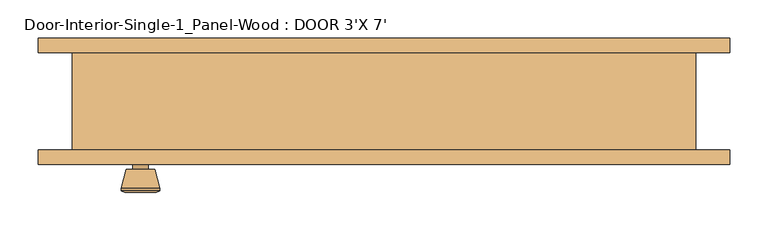
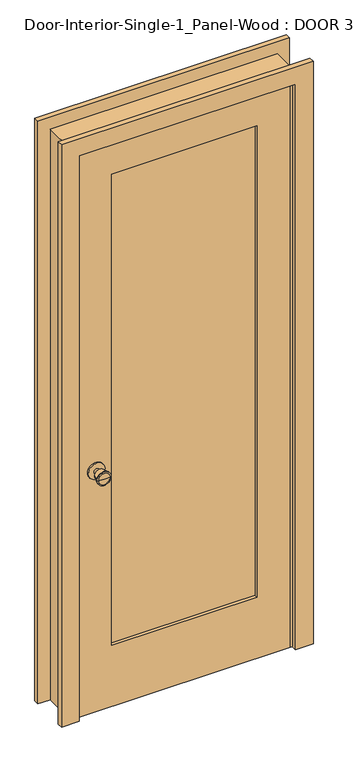
"""IFC4 building model written with IfcOpenShell, lengths in millimetres: door geometry, Door-Interior-Single-1_Panel-Wood : DOOR 3'X 7'."""

from ifc_helpers import new_model, si_unit, point, frame, frame_2d, origin, place, context, project, spatial, polyline, circle_curve, trimmed, segment, composite_curve, outline, extrude, faceted_brep, source, transform, mapped, element, save
from ifc_brep_helpers import plane_surface, cylinder_surface, revolved_surface, advanced_brep


def door_interior_single_1_panel_wood_door_3_x_7_fe7a9c6b(model_context):
    return source(origin(), model_context, "Body", "SolidModel", [
        advanced_brep(
        [(-317.5, -19.4, 914.4), (-327.5, -19.4, 914.4), (-307.5, -19.4, 914.4), (-297.0241324, 29.6, 914.4), (-337.9758676, 29.6, 914.4), (-317.5, 29.6, 914.4), (-292.5, 27.7721319, 914.4), (-342.5, 27.7721319, 914.4), (-292.5, 24.3084537, 914.4), (-342.5, 24.3084537, 914.4), (-298.863764, -0.4, 914.4), (-336.136236, -0.4, 914.4), (-307.5, -0.4, 914.4), (-327.5, -0.4, 914.4)],
        [
            (0, 1),
            (1, 2, circle_curve(frame((-317.5, -19.4, 914.4), z_axis=(0.0, -1.0, 0.0), x_axis=(-1.0, 0.0, 0.0)), 10.0)),
            (2, 0),
            (2, 1, circle_curve(frame((-317.5, -19.4, 914.4), z_axis=(0.0, -1.0, 0.0), x_axis=(-1.0, 0.0, 0.0)), 10.0)),
            (3, 4, circle_curve(frame((-317.5, 29.6, 914.4), z_axis=(0.0, 1.0, 0.0), x_axis=(-1.0, 0.0, 0.0)), 20.4758676)),
            (4, 5),
            (5, 3),
            (4, 3, circle_curve(frame((-317.5, 29.6, 914.4), z_axis=(0.0, 1.0, 0.0), x_axis=(-1.0, 0.0, 0.0)), 20.4758676)),
            (6, 7, circle_curve(frame((-317.5, 27.7721319, 914.4), z_axis=(0.0, 1.0, 0.0), x_axis=(-1.0, 0.0, 0.0)), 25.0)),
            (7, 4),
            (3, 6),
            (7, 6, circle_curve(frame((-317.5, 27.7721319, 914.4), z_axis=(0.0, 1.0, 0.0), x_axis=(-1.0, 0.0, 0.0)), 25.0)),
            (8, 9, circle_curve(frame((-317.5, 24.3084537, 914.4), z_axis=(0.0, 1.0, 0.0), x_axis=(-1.0, 0.0, 0.0)), 25.0)),
            (9, 7),
            (6, 8),
            (9, 8, circle_curve(frame((-317.5, 24.3084537, 914.4), z_axis=(0.0, 1.0, 0.0), x_axis=(-1.0, 0.0, 0.0)), 25.0)),
            (10, 11, circle_curve(frame((-317.5, -0.4, 914.4), z_axis=(0.0, 1.0, 0.0), x_axis=(-1.0, 0.0, 0.0)), 18.636236)),
            (11, 9),
            (8, 10),
            (11, 10, circle_curve(frame((-317.5, -0.4, 914.4), z_axis=(0.0, 1.0, 0.0), x_axis=(-1.0, 0.0, 0.0)), 18.636236)),
            (12, 13, circle_curve(frame((-317.5, -0.4, 914.4), z_axis=(0.0, 1.0, 0.0), x_axis=(-1.0, 0.0, 0.0)), 10.0)),
            (13, 11),
            (10, 12),
            (13, 12, circle_curve(frame((-317.5, -0.4, 914.4), z_axis=(0.0, 1.0, 0.0), x_axis=(-1.0, 0.0, 0.0)), 10.0)),
            (1, 13),
            (12, 2),
        ],
        [
            plane_surface(frame((-317.5, -19.4, 914.4), z_axis=(0.0, -1.0, 0.0), x_axis=(-1.0, 0.0, 0.0))),
            plane_surface(frame((-317.5, 29.6, 914.4), z_axis=(0.0, 1.0, 0.0), x_axis=(-1.0, 0.0, 0.0))),
            revolved_surface(polyline([(-337.9758676, 29.6, 914.4), (-342.5, 27.7721319, 914.4)]), (-317.5, -19.4, 914.4), (0.0, -1.0, 0.0)),
            cylinder_surface(frame((-317.5, -19.4, 914.4), z_axis=(0.0, -1.0, 0.0), x_axis=(-1.0, 0.0, 0.0)), 25.0),
            revolved_surface(polyline([(-342.5, 24.3084537, 914.4), (-336.136236, -0.4, 914.4)]), (-317.5, -19.4, 914.4), (0.0, -1.0, 0.0)),
            plane_surface(frame((-317.5, -0.4, 914.4), z_axis=(0.0, -1.0, 0.0), x_axis=(-1.0, 0.0, 0.0))),
            cylinder_surface(frame((-317.5, -19.4, 914.4), z_axis=(0.0, -1.0, 0.0), x_axis=(-1.0, 0.0, 0.0)), 10.0),
        ],
        [
            (0, [[1, 2, 3]]),
            (0, [[-3, 4, -1]]),
            (1, [[5, 6, 7]]),
            (1, [[8, -7, -6]]),
            (2, [[9, 10, -5, 11]]),
            (2, [[12, -11, -8, -10]]),
            (3, [[13, 14, -9, 15]]),
            (3, [[16, -15, -12, -14]]),
            (4, [[17, 18, -13, 19]]),
            (4, [[20, -19, -16, -18]]),
            (5, [[21, 22, -17, 23]]),
            (5, [[24, -23, -20, -22]]),
            (6, [[-2, 25, -21, 26]]),
            (6, [[-4, -26, -24, -25]]),
        ],
    ),
        extrude(outline(composite_curve([segment(trimmed(circle_curve(frame_2d((914.4, -317.5)), 30.0), [point((914.4, -347.5))], [point((914.4, -287.5))], False, "CARTESIAN"), True, "CONTINUOUS"), segment(trimmed(circle_curve(frame_2d((914.4, -317.5)), 30.0), [point((914.4, -287.5))], [point((914.4, -347.5))], False, "CARTESIAN"), True, "CONTINUOUS")], self_intersect=False)), frame((0.0, -25.4, 0.0), z_axis=(0.0, 1.0, 0.0), x_axis=(0.0, 0.0, 1.0)), (0.0, 0.0, 1.0), 6.0),
        advanced_brep(
        [(-317.5, -66.325, 914.4), (-307.5, -66.325, 914.4), (-327.5, -66.325, 914.4), (-297.0241324, -115.325, 914.4), (-317.5, -115.325, 914.4), (-337.9758676, -115.325, 914.4), (-292.5, -113.4971319, 914.4), (-342.5, -113.4971319, 914.4), (-292.5, -110.0334537, 914.4), (-342.5, -110.0334537, 914.4), (-298.863764, -85.325, 914.4), (-336.136236, -85.325, 914.4), (-307.5, -85.325, 914.4), (-327.5, -85.325, 914.4)],
        [
            (0, 1),
            (1, 2, circle_curve(frame((-317.5, -66.325, 914.4), z_axis=(0.0, 1.0, 0.0), x_axis=(-1.0, 0.0, 0.0)), 10.0)),
            (2, 0),
            (2, 1, circle_curve(frame((-317.5, -66.325, 914.4), z_axis=(0.0, 1.0, 0.0), x_axis=(-1.0, 0.0, 0.0)), 10.0)),
            (3, 4),
            (4, 5),
            (5, 3, circle_curve(frame((-317.5, -115.325, 914.4), z_axis=(0.0, -1.0, 0.0), x_axis=(-1.0, 0.0, 0.0)), 20.4758676)),
            (3, 5, circle_curve(frame((-317.5, -115.325, 914.4), z_axis=(0.0, -1.0, 0.0), x_axis=(-1.0, 0.0, 0.0)), 20.4758676)),
            (6, 3),
            (5, 7),
            (7, 6, circle_curve(frame((-317.5, -113.4971319, 914.4), z_axis=(0.0, -1.0, 0.0), x_axis=(-1.0, 0.0, 0.0)), 25.0)),
            (6, 7, circle_curve(frame((-317.5, -113.4971319, 914.4), z_axis=(0.0, -1.0, 0.0), x_axis=(-1.0, 0.0, 0.0)), 25.0)),
            (8, 6),
            (7, 9),
            (9, 8, circle_curve(frame((-317.5, -110.0334537, 914.4), z_axis=(0.0, -1.0, 0.0), x_axis=(-1.0, 0.0, 0.0)), 25.0)),
            (8, 9, circle_curve(frame((-317.5, -110.0334537, 914.4), z_axis=(0.0, -1.0, 0.0), x_axis=(-1.0, 0.0, 0.0)), 25.0)),
            (10, 8),
            (9, 11),
            (11, 10, circle_curve(frame((-317.5, -85.325, 914.4), z_axis=(0.0, -1.0, 0.0), x_axis=(-1.0, 0.0, 0.0)), 18.636236)),
            (10, 11, circle_curve(frame((-317.5, -85.325, 914.4), z_axis=(0.0, -1.0, 0.0), x_axis=(-1.0, 0.0, 0.0)), 18.636236)),
            (12, 10),
            (11, 13),
            (13, 12, circle_curve(frame((-317.5, -85.325, 914.4), z_axis=(0.0, -1.0, 0.0), x_axis=(-1.0, 0.0, 0.0)), 10.0)),
            (12, 13, circle_curve(frame((-317.5, -85.325, 914.4), z_axis=(0.0, -1.0, 0.0), x_axis=(-1.0, 0.0, 0.0)), 10.0)),
            (1, 12),
            (13, 2),
        ],
        [
            plane_surface(frame((-317.5, -66.325, 914.4), z_axis=(0.0, 1.0, 0.0), x_axis=(-1.0, 0.0, 0.0))),
            plane_surface(frame((-317.5, -115.325, 914.4), z_axis=(0.0, -1.0, 0.0), x_axis=(-1.0, 0.0, 0.0))),
            revolved_surface(polyline([(-337.9758676, -115.325, 914.4), (-342.5, -113.4971319, 914.4)]), (-317.5, -66.325, 914.4), (0.0, 1.0, 0.0)),
            cylinder_surface(frame((-317.5, -66.325, 914.4), z_axis=(0.0, 1.0, 0.0), x_axis=(-1.0, 0.0, 0.0)), 25.0),
            revolved_surface(polyline([(-342.5, -110.0334537, 914.4), (-336.136236, -85.325, 914.4)]), (-317.5, -66.325, 914.4), (0.0, 1.0, 0.0)),
            plane_surface(frame((-317.5, -85.325, 914.4), z_axis=(0.0, 1.0, 0.0), x_axis=(-1.0, 0.0, 0.0))),
            cylinder_surface(frame((-317.5, -66.325, 914.4), z_axis=(0.0, 1.0, 0.0), x_axis=(-1.0, 0.0, 0.0)), 10.0),
        ],
        [
            (0, [[1, 2, 3]]),
            (0, [[-3, 4, -1]]),
            (1, [[5, 6, 7]]),
            (1, [[-6, -5, 8]]),
            (2, [[9, -7, 10, 11]]),
            (2, [[-10, -8, -9, 12]]),
            (3, [[13, -11, 14, 15]]),
            (3, [[-14, -12, -13, 16]]),
            (4, [[17, -15, 18, 19]]),
            (4, [[-18, -16, -17, 20]]),
            (5, [[21, -19, 22, 23]]),
            (5, [[-22, -20, -21, 24]]),
            (6, [[25, -23, 26, -2]]),
            (6, [[-26, -24, -25, -4]]),
        ],
    ),
        extrude(outline(composite_curve([segment(trimmed(circle_curve(frame_2d((914.4, -317.5)), 30.0), [point((914.4, -347.5))], [point((914.4, -287.5))], False, "CARTESIAN"), True, "CONTINUOUS"), segment(trimmed(circle_curve(frame_2d((914.4, -317.5)), 30.0), [point((914.4, -287.5))], [point((914.4, -347.5))], False, "CARTESIAN"), True, "CONTINUOUS")], self_intersect=False)), frame((0.0, -66.325, 0.0), z_axis=(0.0, 1.0, 0.0), x_axis=(0.0, 0.0, 1.0)), (0.0, 0.0, 1.0), 6.0),
        faceted_brep([(406.4, -60.325, 0.0), (381.0, -60.325, 0.0), (381.0, -25.4, 0.0), (368.3, -25.4, 0.0), (368.3, 9.525, 0.0), (381.0, 9.525, 0.0), (381.0, 66.675, 0.0), (406.4, 66.675, 0.0), (406.4, 66.675, 2159.0), (406.4, -60.325, 2159.0), (381.0, 66.675, 2133.6), (-381.0, 66.675, 2133.6), (-381.0, 66.675, 0.0), (-406.4, 66.675, 0.0), (-406.4, 66.675, 2159.0), (381.0, 9.525, 2133.6), (368.3, 9.525, 2120.9), (-368.3, 9.525, 2120.9), (-368.3, 9.525, 0.0), (-381.0, 9.525, 0.0), (-381.0, 9.525, 2133.6), (368.3, -25.4, 2120.9), (381.0, -25.4, 2133.6), (-381.0, -25.4, 2133.6), (-381.0, -25.4, 0.0), (-368.3, -25.4, 0.0), (-368.3, -25.4, 2120.9), (381.0, -60.325, 2133.6), (-406.4, -60.325, 2159.0), (-406.4, -60.325, 0.0), (-381.0, -60.325, 0.0), (-381.0, -60.325, 2133.6)], [[[0, 1, 2, 3, 4, 5, 6, 7]], [[7, 8, 9, 0]], [[6, 10, 11, 12, 13, 14, 8, 7]], [[5, 15, 10, 6]], [[4, 16, 17, 18, 19, 20, 15, 5]], [[3, 21, 16, 4]], [[2, 22, 23, 24, 25, 26, 21, 3]], [[1, 27, 22, 2]], [[0, 9, 28, 29, 30, 31, 27, 1]], [[8, 14, 28, 9]], [[15, 20, 11, 10]], [[21, 26, 17, 16]], [[27, 31, 23, 22]], [[29, 13, 12, 19, 18, 25, 24, 30]], [[14, 13, 29, 28]], [[20, 19, 12, 11]], [[26, 25, 18, 17]], [[31, 30, 24, 23]]]),
        extrude(outline(polyline([(2133.6, -381.0), (0.0, -381.0), (0.0, 381.0), (2133.6, 381.0), (2133.6, -381.0)]), holes=[polyline([(2014.5375, -260.35), (2014.5375, 260.35), (231.775, 260.35), (231.775, -260.35), (2014.5375, -260.35)])]), frame((0.0, -60.325, 0.0), z_axis=(0.0, 1.0, 0.0), x_axis=(0.0, 0.0, 1.0)), (0.0, 0.0, 1.0), 34.925),
        extrude(outline(polyline([(260.35, -37.0416667), (260.35, -48.6833333), (-260.35, -48.6833333), (-260.35, -37.0416667), (260.35, -37.0416667)])), frame((0.0, 0.0, 231.775), z_axis=(0.0, 0.0, 1.0), x_axis=(1.0, 0.0, 0.0)), (0.0, 0.0, 1.0), 1782.7625),
        extrude(outline(polyline([(0.0, 450.85), (2203.45, 450.85), (2203.45, -450.85), (0.0, -450.85), (0.0, -387.35), (2139.95, -387.35), (2139.95, 387.35), (0.0, 387.35), (0.0, 450.85)])), frame((0.0, -79.375, 0.0), z_axis=(0.0, 1.0, 0.0), x_axis=(0.0, 0.0, 1.0)), (0.0, 0.0, 1.0), 19.05),
        extrude(outline(polyline([(0.0, 450.85), (2203.45, 450.85), (2203.45, -450.85), (0.0, -450.85), (0.0, -387.35), (2139.95, -387.35), (2139.95, 387.35), (0.0, 387.35), (0.0, 450.85)])), frame((0.0, 66.675, 0.0), z_axis=(0.0, 1.0, 0.0), x_axis=(0.0, 0.0, 1.0)), (0.0, 0.0, 1.0), 19.05),
    ])


if __name__ == "__main__":
    model = new_model("IFC4")
    model_context = context("Model", 3, world=origin())
    ifc_project = project(units=[si_unit("LENGTHUNIT", "METRE", prefix="MILLI")], contexts=[model_context])
    site = spatial("IfcSite", under=ifc_project)
    building = spatial("IfcBuilding", under=site)
    placement = place(None, origin())
    door_interior_single_1_panel_wood_door_3_x_7_shape = door_interior_single_1_panel_wood_door_3_x_7_fe7a9c6b(model_context)
    element("IfcDoor", 1, ObjectType="Door-Interior-Single-1_Panel-Wood : DOOR 3'X 7'", at=placement, inside=building, context=model_context, shape_type="MappedRepresentation", body=[
        mapped(door_interior_single_1_panel_wood_door_3_x_7_shape, transform((0.0, 0.0, 0.0), x_axis=(1.0, 0.0, 0.0), y_axis=(0.0, 1.0, 0.0), z_axis=(0.0, 0.0, 1.0))),
    ])
    save(model, "model.ifc")

# Revit data of these elements
# Type "Door-Interior-Single-1_Panel-Wood : DOOR 3'X 7'"
#   Type Mark = "11"
#   Assembly Code = "C1020300"
#   Analytic Construction = "Wooden"
#   Top Rail = 0' - 4 11/16"
#   Thickness = 0' - 1 3/8"
#   Thermal Resistance (R) = 2.5876 (h·ft²·°F)/BTU
#   Swing Angle [instance default] = 90.00°
#   Stiles = 0' - 4 3/4"
#   Rough Width = 2' - 8"
#   Rough Height = 7' - 1"
#   Height = 7' - 0"
#   Width = 2' - 6"
#   Heat Transfer Coefficient (U) = 0.3865 BTU/(h·ft²·°F)
#   Bottom Rail = 0' - 9 1/8"
#   Trim Material = Cherry
#   Panel Material = Cherry
#   Frame Material = Cherry
#   Door Handle Material = Aluminum
#   Visual Light Transmittance = 0
#   Solar Heat Gain Coefficient = 0
#   Wall Closure = (empty or 0)
#   Function = (empty or 0)
# Element 1 (IfcDoor, "Door-Interior-Single-1_Panel-Wood : DOOR 3'X 7'")
#   Materials on its faces: "Cherry", "Aluminum"
# Materials
#   "Cherry": class "Wood", colour RGB 226 177 128, transparency 0, Description = "Prunus Serotina", Cost = 0
#   "Aluminum": class "Metal", colour RGB 247 247 247, transparency 0, Description = "Aluminum 6061", Cost = 0
